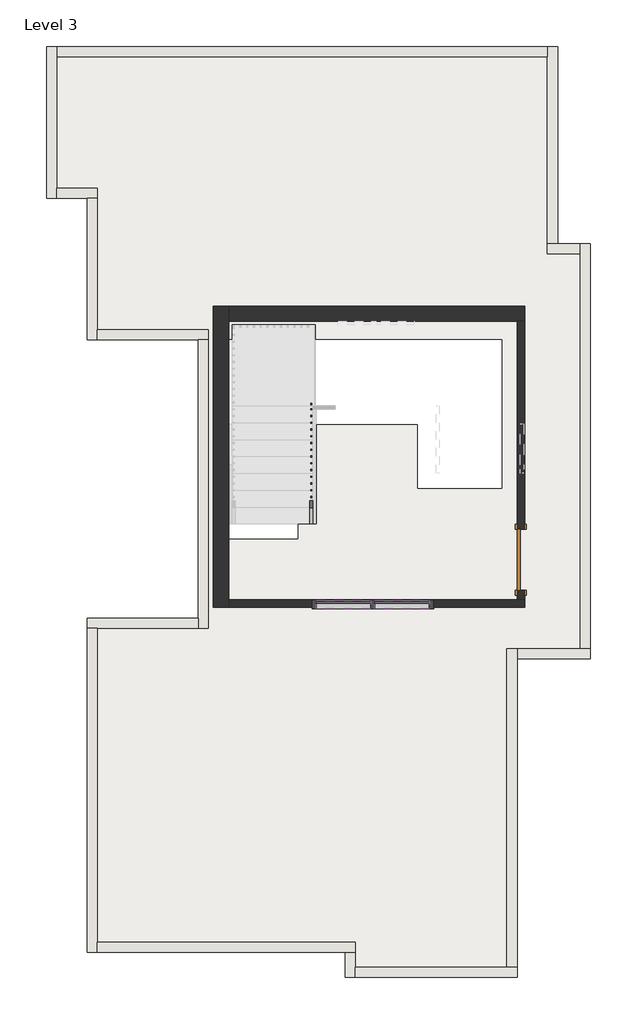
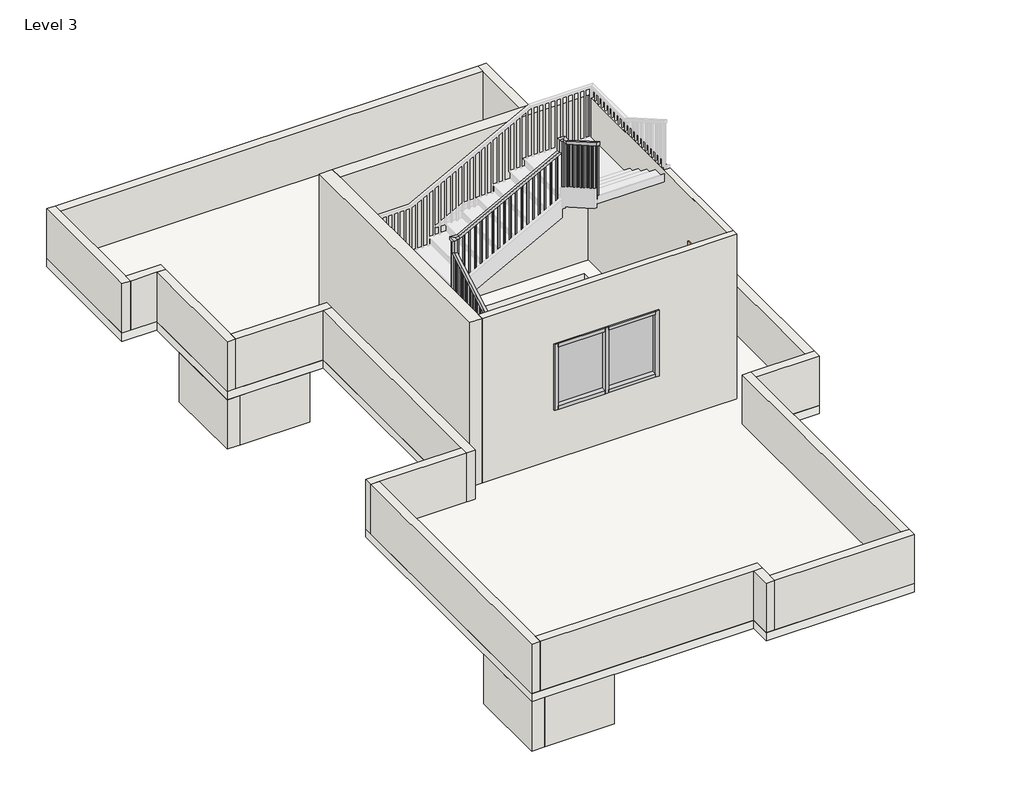
# One storey, part 1 of 2: 24 walls, 7 members, 2 plates, 1 door, 1 railing, 1 roof.
"""IFC4 building model written with IfcOpenShell, lengths in millimetres."""

from ifc_helpers import new_model, si_unit, frame, origin, place, context, project, spatial, polyline, outline, extrude, faceted_brep, transform, mapped, element, save
from components import single_flush_door_3_305aa2a5, member_75074519, member_2b49869a, member_c17f1be2, system_panel_glazed_d6173012

model = new_model("IFC4")

# Units and contexts
model_context = context("Model", 3, world=origin())
ifc_project = project(units=[si_unit("LENGTHUNIT", "METRE", prefix="MILLI")], contexts=[model_context])

# Site, building, storey
site = spatial("IfcSite", under=ifc_project)
building = spatial("IfcBuilding", under=site)
storey = spatial("IfcBuildingStorey", under=building, Name="Level 3", Elevation=6248.4)

# Door
placement = place(None, origin())
single_flush_door_3_shape = single_flush_door_3_305aa2a5(model_context)
element("IfcDoor", 1, ObjectType="Single-Flush : door 3'", at=placement, inside=storey, context=model_context, shape_type="MappedRepresentation", body=[
    mapped(single_flush_door_3_shape, transform((-36373.0566834, 12147.2118061, 6248.4), x_axis=(0.0, -1.0, 0.0), y_axis=(1.0, 0.0, 0.0), z_axis=(0.0, 0.0, 1.0))),
])

# Members
member_shape = member_75074519(model_context)
element("IfcMember", 2, ObjectType="Rectangular Mullion : 2.5\" x 5\" rectangular", at=placement, inside=storey, context=model_context, shape_type="MappedRepresentation", body=[
    mapped(member_shape, transform((-37687.5066834, 11472.9643297, 7162.8), x_axis=(1.0, 0.0, 0.0), y_axis=(0.0, -1.0, 0.0), z_axis=(0.0, 0.0, -1.0))),
])
element("IfcMember", 3, ObjectType="Rectangular Mullion : 2.5\" x 5\" rectangular", at=placement, inside=storey, context=model_context, shape_type="MappedRepresentation", body=[
    mapped(member_shape, transform((-39516.3066834, 11472.9643297, 8382.0), x_axis=(-1.0, 0.0, 0.0), y_axis=(0.0, -1.0, 0.0), z_axis=(0.0, 0.0, 1.0))),
])
member_2_shape = member_2b49869a(model_context)
element("IfcMember", 4, ObjectType="Rectangular Mullion : 2.5\" x 5\" rectangular", at=placement, inside=storey, context=model_context, shape_type="MappedRepresentation", body=[
    mapped(member_2_shape, transform((-38601.9066834, 11472.9643297, 7162.8), x_axis=(1.0, 0.0, 0.0), y_axis=(0.0, -1.0, 0.0), z_axis=(0.0, 0.0, -1.0))),
])
member_3_shape = member_c17f1be2(model_context)
element("IfcMember", 5, ObjectType="Rectangular Mullion : 2.5\" x 5\" rectangular", at=placement, inside=storey, context=model_context, shape_type="MappedRepresentation", body=[
    mapped(member_3_shape, transform((-37751.0066834, 11472.9643297, 8382.0), x_axis=(0.0, 0.0, 1.0), y_axis=(0.0, -1.0, 0.0), z_axis=(1.0, 0.0, 0.0))),
])
element("IfcMember", 6, ObjectType="Rectangular Mullion : 2.5\" x 5\" rectangular", at=placement, inside=storey, context=model_context, shape_type="MappedRepresentation", body=[
    mapped(member_3_shape, transform((-38633.6566834, 11472.9643297, 8382.0), x_axis=(0.0, 0.0, 1.0), y_axis=(0.0, -1.0, 0.0), z_axis=(1.0, 0.0, 0.0))),
])
element("IfcMember", 7, ObjectType="Rectangular Mullion : 2.5\" x 5\" rectangular", at=placement, inside=storey, context=model_context, shape_type="MappedRepresentation", body=[
    mapped(member_3_shape, transform((-39452.8066834, 11472.9643297, 7162.8), x_axis=(0.0, 0.0, -1.0), y_axis=(0.0, -1.0, 0.0), z_axis=(-1.0, 0.0, 0.0))),
])
element("IfcMember", 8, ObjectType="Rectangular Mullion : 2.5\" x 5\" rectangular", at=placement, inside=storey, context=model_context, shape_type="MappedRepresentation", body=[
    mapped(member_3_shape, transform((-38570.1566834, 11472.9643297, 7162.8), x_axis=(0.0, 0.0, -1.0), y_axis=(0.0, -1.0, 0.0), z_axis=(-1.0, 0.0, 0.0))),
])

# Plates
system_panel_glazed_shape = system_panel_glazed_d6173012(model_context)
element("IfcPlate", 9, ObjectType="System Panel : Glazed", at=placement, inside=storey, context=model_context, shape_type="MappedRepresentation", body=[
    mapped(system_panel_glazed_shape, transform((-39043.2316834, 11472.9643297, 7226.3), x_axis=(1.0, 0.0, 0.0), y_axis=(0.0, 1.0, 0.0), z_axis=(0.0, 0.0, 1.0))),
])
element("IfcPlate", 10, ObjectType="System Panel : Glazed", at=placement, inside=storey, context=model_context, shape_type="MappedRepresentation", body=[
    mapped(system_panel_glazed_shape, transform((-38160.5816834, 11472.9643297, 7226.3), x_axis=(1.0, 0.0, 0.0), y_axis=(0.0, 1.0, 0.0), z_axis=(0.0, 0.0, 1.0))),
])

# Railing
element("IfcRailing", 11, ObjectType="Handrail - Rectangular", at=placement, inside=storey, context=model_context, shape_type="SolidModel", body=[
    faceted_brep([(-39553.9146233, 12686.9618061, 7307.9428571), (-39553.9146233, 12686.9618061, 7249.4339009), (-39503.1146233, 12686.9618061, 7249.4339009), (-39503.1146233, 12686.9618061, 7307.9428571), (-39553.9146233, 14388.7618061, 8280.4), (-39553.9146233, 14439.5618061, 8250.9196152), (-39503.1146233, 14439.5618061, 8250.9196152), (-39503.1146233, 14388.7618061, 8280.4), (-39553.9146233, 14388.7618061, 8509.7257143), (-39553.9146233, 14439.5618061, 8458.9257143), (-39503.1146233, 14439.5618061, 8458.9257143), (-39503.1146233, 14388.7618061, 8509.7257143), (-39553.9146233, 14515.7618061, 8509.7257143), (-39553.9146233, 14515.7618061, 8458.9257143), (-39503.1146233, 14464.9618061, 8458.9257143), (-39503.1146233, 14464.9618061, 8509.7257143), (-39426.9146233, 14515.7618061, 8509.7257143), (-39414.2146233, 14515.7618061, 8458.9257143), (-39414.2146233, 14464.9618061, 8458.9257143), (-39426.9146233, 14464.9618061, 8509.7257143), (-37674.3146233, 14515.7618061, 9444.4457143), (-37623.5146233, 14515.7618061, 9413.9657143), (-37623.5146233, 14464.9618061, 9413.9657143), (-37674.3146233, 14464.9618061, 9444.4457143), (-37674.3146233, 14515.7618061, 9673.7714286), (-37623.5146233, 14515.7618061, 9622.9714286), (-37623.5146233, 14464.9618061, 9622.9714286), (-37674.3146233, 14464.9618061, 9673.7714286), (-37547.3146233, 14515.7618061, 9673.7714286), (-37547.3146233, 14515.7618061, 9622.9714286), (-37598.1146233, 14464.9618061, 9622.9714286), (-37598.1146233, 14464.9618061, 9673.7714286), (-37547.3146233, 14388.7618061, 9673.7714286), (-37547.3146233, 14375.2711327, 9622.9714286), (-37598.1146233, 14375.2711327, 9622.9714286), (-37598.1146233, 14388.7618061, 9673.7714286), (-37547.3146233, 13448.9618061, 10210.8), (-37598.1146233, 13448.9618061, 10210.8), (-37598.1146233, 13448.9618061, 10152.2910438), (-37547.3146233, 13448.9618061, 10152.2910438)], [[[0, 1, 2, 3]], [[1, 0, 4, 5]], [[2, 1, 5, 6]], [[3, 2, 6, 7]], [[0, 3, 7, 4]], [[5, 4, 8, 9]], [[6, 5, 9, 10]], [[7, 6, 10, 11]], [[4, 7, 11, 8]], [[9, 8, 12, 13]], [[10, 9, 13, 14]], [[11, 10, 14, 15]], [[8, 11, 15, 12]], [[13, 12, 16, 17]], [[14, 13, 17, 18]], [[15, 14, 18, 19]], [[12, 15, 19, 16]], [[17, 16, 20, 21]], [[18, 17, 21, 22]], [[19, 18, 22, 23]], [[16, 19, 23, 20]], [[21, 20, 24, 25]], [[22, 21, 25, 26]], [[23, 22, 26, 27]], [[20, 23, 27, 24]], [[25, 24, 28, 29]], [[26, 25, 29, 30]], [[27, 26, 30, 31]], [[24, 27, 31, 28]], [[29, 28, 32, 33]], [[30, 29, 33, 34]], [[31, 30, 34, 35]], [[28, 31, 35, 32]], [[36, 37, 38, 39]], [[33, 32, 36, 39]], [[34, 33, 39, 38]], [[35, 34, 38, 37]], [[32, 35, 37, 36]]]),
    extrude(outline(polyline([(13464.8368061, 10143.2196152), (13483.8868061, 10132.3339009), (13483.8868061, 9151.2571429), (13464.8368061, 9151.2571429), (13464.8368061, 10143.2196152)])), frame((-37582.2396233, 0.0, 0.0), z_axis=(1.0, 0.0, 0.0), x_axis=(0.0, 1.0, 0.0)), (0.0, 0.0, 1.0), 19.05),
    extrude(outline(polyline([(13566.4368061, 10085.1624723), (13585.4868061, 10074.2767581), (13585.4868061, 9151.2571429), (13566.4368061, 9151.2571429), (13566.4368061, 10085.1624723)])), frame((-37582.2396233, 0.0, 0.0), z_axis=(1.0, 0.0, 0.0), x_axis=(0.0, 1.0, 0.0)), (0.0, 0.0, 1.0), 19.05),
    extrude(outline(polyline([(13668.0368061, 10027.1053295), (13687.0868061, 10016.2196152), (13687.0868061, 9151.2571429), (13668.0368061, 9151.2571429), (13668.0368061, 10027.1053295)])), frame((-37582.2396233, 0.0, 0.0), z_axis=(1.0, 0.0, 0.0), x_axis=(0.0, 1.0, 0.0)), (0.0, 0.0, 1.0), 19.05),
    extrude(outline(polyline([(13769.6368061, 9969.0481866), (13788.6868061, 9958.1624723), (13788.6868061, 9006.1142857), (13769.6368061, 9006.1142857), (13769.6368061, 9969.0481866)])), frame((-37582.2396233, 0.0, 0.0), z_axis=(1.0, 0.0, 0.0), x_axis=(0.0, 1.0, 0.0)), (0.0, 0.0, 1.0), 19.05),
    extrude(outline(polyline([(13871.2368061, 9910.9910438), (13890.2868061, 9900.1053295), (13890.2868061, 9006.1142857), (13871.2368061, 9006.1142857), (13871.2368061, 9910.9910438)])), frame((-37582.2396233, 0.0, 0.0), z_axis=(1.0, 0.0, 0.0), x_axis=(0.0, 1.0, 0.0)), (0.0, 0.0, 1.0), 19.05),
    extrude(outline(polyline([(13972.8368061, 9852.9339009), (13991.8868061, 9842.0481866), (13991.8868061, 8860.9714286), (13972.8368061, 8860.9714286), (13972.8368061, 9852.9339009)])), frame((-37582.2396233, 0.0, 0.0), z_axis=(1.0, 0.0, 0.0), x_axis=(0.0, 1.0, 0.0)), (0.0, 0.0, 1.0), 19.05),
    extrude(outline(polyline([(14074.4368061, 9794.8767581), (14093.4868061, 9783.9910438), (14093.4868061, 8860.9714286), (14074.4368061, 8860.9714286), (14074.4368061, 9794.8767581)])), frame((-37582.2396233, 0.0, 0.0), z_axis=(1.0, 0.0, 0.0), x_axis=(0.0, 1.0, 0.0)), (0.0, 0.0, 1.0), 19.05),
    extrude(outline(polyline([(14176.0368061, 9736.8196152), (14195.0868061, 9725.9339009), (14195.0868061, 8860.9714286), (14176.0368061, 8860.9714286), (14176.0368061, 9736.8196152)])), frame((-37582.2396233, 0.0, 0.0), z_axis=(1.0, 0.0, 0.0), x_axis=(0.0, 1.0, 0.0)), (0.0, 0.0, 1.0), 19.05),
    extrude(outline(polyline([(14277.6368061, 9678.7624723), (14296.6868061, 9667.8767581), (14296.6868061, 8715.8285714), (14277.6368061, 8715.8285714), (14277.6368061, 9678.7624723)])), frame((-37582.2396233, 0.0, 0.0), z_axis=(1.0, 0.0, 0.0), x_axis=(0.0, 1.0, 0.0)), (0.0, 0.0, 1.0), 19.05),
    extrude(outline(polyline([(14379.2368061, 9620.7053295), (14398.2868061, 9609.8196152), (14398.2868061, 8715.8285714), (14379.2368061, 8715.8285714), (14379.2368061, 9620.7053295)])), frame((-37582.2396233, 0.0, 0.0), z_axis=(1.0, 0.0, 0.0), x_axis=(0.0, 1.0, 0.0)), (0.0, 0.0, 1.0), 19.05),
    extrude(outline(polyline([(-37607.6396233, 14480.8368061), (-37607.6396233, 14499.8868061), (-37588.5896233, 14499.8868061), (-37588.5896233, 14480.8368061), (-37607.6396233, 14480.8368061)])), frame((0.0, 0.0, 8570.6857143), z_axis=(0.0, 0.0, 1.0), x_axis=(1.0, 0.0, 0.0)), (0.0, 0.0, 1.0), 1052.2857143),
    extrude(outline(polyline([(9378.4057143, -37690.1896233), (9368.2457143, -37709.2396233), (8425.5428571, -37709.2396233), (8425.5428571, -37690.1896233), (9378.4057143, -37690.1896233)])), frame((0.0, 14480.8368061, 0.0), z_axis=(0.0, 1.0, 0.0), x_axis=(0.0, 0.0, 1.0)), (0.0, 0.0, 1.0), 19.05),
    extrude(outline(polyline([(9324.2190476, -37791.7896233), (9314.0590476, -37810.8396233), (8425.5428571, -37810.8396233), (8425.5428571, -37791.7896233), (9324.2190476, -37791.7896233)])), frame((0.0, 14480.8368061, 0.0), z_axis=(0.0, 1.0, 0.0), x_axis=(0.0, 0.0, 1.0)), (0.0, 0.0, 1.0), 19.05),
    extrude(outline(polyline([(9270.032381, -37893.3896233), (9259.872381, -37912.4396233), (8280.4, -37912.4396233), (8280.4, -37893.3896233), (9270.032381, -37893.3896233)])), frame((0.0, 14480.8368061, 0.0), z_axis=(0.0, 1.0, 0.0), x_axis=(0.0, 0.0, 1.0)), (0.0, 0.0, 1.0), 19.05),
    extrude(outline(polyline([(9215.8457143, -37994.9896233), (9205.6857143, -38014.0396233), (8280.4, -38014.0396233), (8280.4, -37994.9896233), (9215.8457143, -37994.9896233)])), frame((0.0, 14480.8368061, 0.0), z_axis=(0.0, 1.0, 0.0), x_axis=(0.0, 0.0, 1.0)), (0.0, 0.0, 1.0), 19.05),
    extrude(outline(polyline([(9161.6590476, -38096.5896233), (9151.4990476, -38115.6396233), (8280.4, -38115.6396233), (8280.4, -38096.5896233), (9161.6590476, -38096.5896233)])), frame((0.0, 14480.8368061, 0.0), z_axis=(0.0, 1.0, 0.0), x_axis=(0.0, 0.0, 1.0)), (0.0, 0.0, 1.0), 19.05),
    extrude(outline(polyline([(9107.472381, -38198.1896233), (9097.312381, -38217.2396233), (8135.2571429, -38217.2396233), (8135.2571429, -38198.1896233), (9107.472381, -38198.1896233)])), frame((0.0, 14480.8368061, 0.0), z_axis=(0.0, 1.0, 0.0), x_axis=(0.0, 0.0, 1.0)), (0.0, 0.0, 1.0), 19.05),
    extrude(outline(polyline([(9053.2857143, -38299.7896233), (9043.1257143, -38318.8396233), (8135.2571429, -38318.8396233), (8135.2571429, -38299.7896233), (9053.2857143, -38299.7896233)])), frame((0.0, 14480.8368061, 0.0), z_axis=(0.0, 1.0, 0.0), x_axis=(0.0, 0.0, 1.0)), (0.0, 0.0, 1.0), 19.05),
    extrude(outline(polyline([(8999.0990476, -38401.3896233), (8988.9390476, -38420.4396233), (8135.2571429, -38420.4396233), (8135.2571429, -38401.3896233), (8999.0990476, -38401.3896233)])), frame((0.0, 14480.8368061, 0.0), z_axis=(0.0, 1.0, 0.0), x_axis=(0.0, 0.0, 1.0)), (0.0, 0.0, 1.0), 19.05),
    extrude(outline(polyline([(8944.912381, -38502.9896233), (8934.752381, -38522.0396233), (7990.1142857, -38522.0396233), (7990.1142857, -38502.9896233), (8944.912381, -38502.9896233)])), frame((0.0, 14480.8368061, 0.0), z_axis=(0.0, 1.0, 0.0), x_axis=(0.0, 0.0, 1.0)), (0.0, 0.0, 1.0), 19.05),
    extrude(outline(polyline([(8890.7257143, -38604.5896233), (8880.5657143, -38623.6396233), (7990.1142857, -38623.6396233), (7990.1142857, -38604.5896233), (8890.7257143, -38604.5896233)])), frame((0.0, 14480.8368061, 0.0), z_axis=(0.0, 1.0, 0.0), x_axis=(0.0, 0.0, 1.0)), (0.0, 0.0, 1.0), 19.05),
    extrude(outline(polyline([(8836.5390476, -38706.1896233), (8826.3790476, -38725.2396233), (7844.9714286, -38725.2396233), (7844.9714286, -38706.1896233), (8836.5390476, -38706.1896233)])), frame((0.0, 14480.8368061, 0.0), z_axis=(0.0, 1.0, 0.0), x_axis=(0.0, 0.0, 1.0)), (0.0, 0.0, 1.0), 19.05),
    extrude(outline(polyline([(8782.352381, -38807.7896233), (8772.192381, -38826.8396233), (7844.9714286, -38826.8396233), (7844.9714286, -38807.7896233), (8782.352381, -38807.7896233)])), frame((0.0, 14480.8368061, 0.0), z_axis=(0.0, 1.0, 0.0), x_axis=(0.0, 0.0, 1.0)), (0.0, 0.0, 1.0), 19.05),
    extrude(outline(polyline([(8728.1657143, -38909.3896233), (8718.0057143, -38928.4396233), (7844.9714286, -38928.4396233), (7844.9714286, -38909.3896233), (8728.1657143, -38909.3896233)])), frame((0.0, 14480.8368061, 0.0), z_axis=(0.0, 1.0, 0.0), x_axis=(0.0, 0.0, 1.0)), (0.0, 0.0, 1.0), 19.05),
    extrude(outline(polyline([(8673.9790476, -39010.9896233), (8663.8190476, -39030.0396233), (7699.8285714, -39030.0396233), (7699.8285714, -39010.9896233), (8673.9790476, -39010.9896233)])), frame((0.0, 14480.8368061, 0.0), z_axis=(0.0, 1.0, 0.0), x_axis=(0.0, 0.0, 1.0)), (0.0, 0.0, 1.0), 19.05),
    extrude(outline(polyline([(8619.792381, -39112.5896233), (8609.632381, -39131.6396233), (7699.8285714, -39131.6396233), (7699.8285714, -39112.5896233), (8619.792381, -39112.5896233)])), frame((0.0, 14480.8368061, 0.0), z_axis=(0.0, 1.0, 0.0), x_axis=(0.0, 0.0, 1.0)), (0.0, 0.0, 1.0), 19.05),
    extrude(outline(polyline([(8565.6057143, -39214.1896233), (8555.4457143, -39233.2396233), (7699.8285714, -39233.2396233), (7699.8285714, -39214.1896233), (8565.6057143, -39214.1896233)])), frame((0.0, 14480.8368061, 0.0), z_axis=(0.0, 1.0, 0.0), x_axis=(0.0, 0.0, 1.0)), (0.0, 0.0, 1.0), 19.05),
    extrude(outline(polyline([(8511.4190476, -39315.7896233), (8501.2590476, -39334.8396233), (7554.6857143, -39334.8396233), (7554.6857143, -39315.7896233), (8511.4190476, -39315.7896233)])), frame((0.0, 14480.8368061, 0.0), z_axis=(0.0, 1.0, 0.0), x_axis=(0.0, 0.0, 1.0)), (0.0, 0.0, 1.0), 19.05),
    extrude(outline(polyline([(8457.232381, -39417.3896233), (8447.072381, -39436.4396233), (7554.6857143, -39436.4396233), (7554.6857143, -39417.3896233), (8457.232381, -39417.3896233)])), frame((0.0, 14480.8368061, 0.0), z_axis=(0.0, 1.0, 0.0), x_axis=(0.0, 0.0, 1.0)), (0.0, 0.0, 1.0), 19.05),
    extrude(outline(polyline([(-39518.9896233, 14404.6368061), (-39538.0396233, 14404.6368061), (-39538.0396233, 14423.6868061), (-39518.9896233, 14423.6868061), (-39518.9896233, 14404.6368061)])), frame((0.0, 0.0, 7264.4), z_axis=(0.0, 0.0, 1.0), x_axis=(1.0, 0.0, 0.0)), (0.0, 0.0, 1.0), 1194.5257143),
    extrude(outline(polyline([(14303.0368061, 8172.9053295), (14322.0868061, 8183.7910438), (14322.0868061, 7264.4), (14303.0368061, 7264.4), (14303.0368061, 8172.9053295)])), frame((-39538.0396233, 0.0, 0.0), z_axis=(1.0, 0.0, 0.0), x_axis=(0.0, 1.0, 0.0)), (0.0, 0.0, 1.0), 19.05),
    extrude(outline(polyline([(14201.4368061, 8114.8481866), (14220.4868061, 8125.7339009), (14220.4868061, 7264.4), (14201.4368061, 7264.4), (14201.4368061, 8114.8481866)])), frame((-39538.0396233, 0.0, 0.0), z_axis=(1.0, 0.0, 0.0), x_axis=(0.0, 1.0, 0.0)), (0.0, 0.0, 1.0), 19.05),
    extrude(outline(polyline([(14099.8368061, 8056.7910438), (14118.8868061, 8067.6767581), (14118.8868061, 7119.2571429), (14099.8368061, 7119.2571429), (14099.8368061, 8056.7910438)])), frame((-39538.0396233, 0.0, 0.0), z_axis=(1.0, 0.0, 0.0), x_axis=(0.0, 1.0, 0.0)), (0.0, 0.0, 1.0), 19.05),
    extrude(outline(polyline([(13998.2368061, 7998.7339009), (14017.2868061, 8009.6196152), (14017.2868061, 7119.2571429), (13998.2368061, 7119.2571429), (13998.2368061, 7998.7339009)])), frame((-39538.0396233, 0.0, 0.0), z_axis=(1.0, 0.0, 0.0), x_axis=(0.0, 1.0, 0.0)), (0.0, 0.0, 1.0), 19.05),
    extrude(outline(polyline([(13896.6368061, 7940.6767581), (13915.6868061, 7951.5624723), (13915.6868061, 6974.1142857), (13896.6368061, 6974.1142857), (13896.6368061, 7940.6767581)])), frame((-39538.0396233, 0.0, 0.0), z_axis=(1.0, 0.0, 0.0), x_axis=(0.0, 1.0, 0.0)), (0.0, 0.0, 1.0), 19.05),
    extrude(outline(polyline([(13795.0368061, 7882.6196152), (13814.0868061, 7893.5053295), (13814.0868061, 6974.1142857), (13795.0368061, 6974.1142857), (13795.0368061, 7882.6196152)])), frame((-39538.0396233, 0.0, 0.0), z_axis=(1.0, 0.0, 0.0), x_axis=(0.0, 1.0, 0.0)), (0.0, 0.0, 1.0), 19.05),
    extrude(outline(polyline([(13693.4368061, 7824.5624723), (13712.4868061, 7835.4481866), (13712.4868061, 6974.1142857), (13693.4368061, 6974.1142857), (13693.4368061, 7824.5624723)])), frame((-39538.0396233, 0.0, 0.0), z_axis=(1.0, 0.0, 0.0), x_axis=(0.0, 1.0, 0.0)), (0.0, 0.0, 1.0), 19.05),
    extrude(outline(polyline([(13591.8368061, 7766.5053295), (13610.8868061, 7777.3910438), (13610.8868061, 6828.9714286), (13591.8368061, 6828.9714286), (13591.8368061, 7766.5053295)])), frame((-39538.0396233, 0.0, 0.0), z_axis=(1.0, 0.0, 0.0), x_axis=(0.0, 1.0, 0.0)), (0.0, 0.0, 1.0), 19.05),
    extrude(outline(polyline([(13490.2368061, 7708.4481866), (13509.2868061, 7719.3339009), (13509.2868061, 6828.9714286), (13490.2368061, 6828.9714286), (13490.2368061, 7708.4481866)])), frame((-39538.0396233, 0.0, 0.0), z_axis=(1.0, 0.0, 0.0), x_axis=(0.0, 1.0, 0.0)), (0.0, 0.0, 1.0), 19.05),
    extrude(outline(polyline([(13388.6368061, 7650.3910438), (13407.6868061, 7661.2767581), (13407.6868061, 6683.8285714), (13388.6368061, 6683.8285714), (13388.6368061, 7650.3910438)])), frame((-39538.0396233, 0.0, 0.0), z_axis=(1.0, 0.0, 0.0), x_axis=(0.0, 1.0, 0.0)), (0.0, 0.0, 1.0), 19.05),
    extrude(outline(polyline([(13287.0368061, 7592.3339009), (13306.0868061, 7603.2196152), (13306.0868061, 6683.8285714), (13287.0368061, 6683.8285714), (13287.0368061, 7592.3339009)])), frame((-39538.0396233, 0.0, 0.0), z_axis=(1.0, 0.0, 0.0), x_axis=(0.0, 1.0, 0.0)), (0.0, 0.0, 1.0), 19.05),
    extrude(outline(polyline([(13185.4368061, 7534.2767581), (13204.4868061, 7545.1624723), (13204.4868061, 6683.8285714), (13185.4368061, 6683.8285714), (13185.4368061, 7534.2767581)])), frame((-39538.0396233, 0.0, 0.0), z_axis=(1.0, 0.0, 0.0), x_axis=(0.0, 1.0, 0.0)), (0.0, 0.0, 1.0), 19.05),
    extrude(outline(polyline([(13083.8368061, 7476.2196152), (13102.8868061, 7487.1053295), (13102.8868061, 6538.6857143), (13083.8368061, 6538.6857143), (13083.8368061, 7476.2196152)])), frame((-39538.0396233, 0.0, 0.0), z_axis=(1.0, 0.0, 0.0), x_axis=(0.0, 1.0, 0.0)), (0.0, 0.0, 1.0), 19.05),
    extrude(outline(polyline([(12982.2368061, 7418.1624723), (13001.2868061, 7429.0481866), (13001.2868061, 6538.6857143), (12982.2368061, 6538.6857143), (12982.2368061, 7418.1624723)])), frame((-39538.0396233, 0.0, 0.0), z_axis=(1.0, 0.0, 0.0), x_axis=(0.0, 1.0, 0.0)), (0.0, 0.0, 1.0), 19.05),
    extrude(outline(polyline([(12880.6368061, 7360.1053295), (12899.6868061, 7370.9910438), (12899.6868061, 6393.5428571), (12880.6368061, 6393.5428571), (12880.6368061, 7360.1053295)])), frame((-39538.0396233, 0.0, 0.0), z_axis=(1.0, 0.0, 0.0), x_axis=(0.0, 1.0, 0.0)), (0.0, 0.0, 1.0), 19.05),
    extrude(outline(polyline([(12779.0368061, 7302.0481866), (12798.0868061, 7312.9339009), (12798.0868061, 6393.5428571), (12779.0368061, 6393.5428571), (12779.0368061, 7302.0481866)])), frame((-39538.0396233, 0.0, 0.0), z_axis=(1.0, 0.0, 0.0), x_axis=(0.0, 1.0, 0.0)), (0.0, 0.0, 1.0), 19.05),
    extrude(outline(polyline([(-37582.2396233, 14480.8368061), (-37582.2396233, 14499.8868061), (-37563.1896233, 14499.8868061), (-37563.1896233, 14480.8368061), (-37582.2396233, 14480.8368061)])), frame((0.0, 0.0, 8570.6857143), z_axis=(0.0, 0.0, 1.0), x_axis=(1.0, 0.0, 0.0)), (0.0, 0.0, 1.0), 1052.2857143),
    extrude(outline(polyline([(-39518.9896233, 14480.8368061), (-39538.0396233, 14480.8368061), (-39538.0396233, 14499.8868061), (-39518.9896233, 14499.8868061), (-39518.9896233, 14480.8368061)])), frame((0.0, 0.0, 7409.5428571), z_axis=(0.0, 0.0, 1.0), x_axis=(1.0, 0.0, 0.0)), (0.0, 0.0, 1.0), 1049.3828571),
    extrude(outline(polyline([(13448.9618061, 10152.2910438), (13468.0118061, 10141.4053295), (13468.0118061, 9151.2571429), (13448.9618061, 9151.2571429), (13448.9618061, 10152.2910438)])), frame((-37582.2396233, 0.0, 0.0), z_axis=(1.0, 0.0, 0.0), x_axis=(0.0, 1.0, 0.0)), (0.0, 0.0, 1.0), 19.05),
    extrude(outline(polyline([(12686.9618061, 7249.4339009), (12706.0118061, 7260.3196152), (12706.0118061, 6393.5428571), (12686.9618061, 6393.5428571), (12686.9618061, 7249.4339009)])), frame((-39538.0396233, 0.0, 0.0), z_axis=(1.0, 0.0, 0.0), x_axis=(0.0, 1.0, 0.0)), (0.0, 0.0, 1.0), 19.05),
])

# Roof
element("IfcRoof", 12, ObjectType="ROOF 6\"", at=placement, inside=storey, context=model_context, shape_type="SweptSolid", body=[
    extrude(outline(polyline([(-42906.7146233, 15456.5864709), (-42906.7146233, 17590.1864709), (-43516.3146233, 17590.1864709), (-43516.3146233, 19876.1864709), (-35820.1146233, 19876.1864709), (-35820.1146233, 16904.3864709), (-35324.8146233, 16904.3864709), (-35324.8146233, 10655.9864709), (-36429.7146233, 10655.9864709), (-36429.7146233, 5855.3080647), (-39020.5146233, 5855.3080647), (-39020.5146233, 6236.3864709), (-42906.7146233, 6236.3864709), (-42906.7146233, 11265.5864709), (-41230.3146233, 11265.5864709), (-41230.3146233, 15456.5864709), (-42906.7146233, 15456.5864709)]), holes=[polyline([(-36658.3146233, 15456.5864709), (-41001.7146233, 15456.5864709), (-41001.7146233, 12459.3864709), (-39731.7146233, 12459.3864709), (-39731.7146233, 14186.5864709), (-37928.3146233, 14186.5864709), (-37928.3146233, 13221.3864709), (-36658.3146233, 13221.3864709), (-36658.3146233, 15456.5864709)])]), frame((0.0, 0.0, 6096.0), z_axis=(0.0, 0.0, 1.0), x_axis=(1.0, 0.0, 0.0)), (0.0, 0.0, 1.0), 152.4),
])

# Walls
element("IfcWall", 13, ObjectType="Generic - 5\"", at=placement, inside=storey, context=model_context, shape_type="Brep", body=[
    faceted_brep([(-40773.1146233, 11429.6618061, 6248.4), (-36315.9066834, 11429.6618061, 6248.4), (-36315.9066834, 11429.6618061, 9296.4), (-40773.1146233, 11429.6618061, 9296.4), (-39516.3066834, 11429.6618061, 7162.8), (-39516.3066834, 11429.6618061, 8382.0), (-37687.5066834, 11429.6618061, 8382.0), (-37687.5066834, 11429.6618061, 7162.8), (-36315.9066834, 11543.9618061, 6248.4), (-36430.2066834, 11543.9618061, 6248.4), (-40773.1146233, 11543.9618061, 6248.4), (-40773.1146233, 11543.9618061, 9296.4), (-36430.2066834, 11543.9618061, 9296.4), (-36315.9066834, 11543.9618061, 9296.4), (-39516.3066834, 11543.9618061, 8382.0), (-39516.3066834, 11543.9618061, 7162.8), (-37687.5066834, 11543.9618061, 7162.8), (-37687.5066834, 11543.9618061, 8382.0)], [[[0, 1, 2, 3], [4, 5, 6, 7]], [[8, 9, 10, 11, 12, 13], [14, 15, 16, 17]], [[1, 0, 10, 9, 8]], [[2, 1, 8, 13]], [[0, 3, 11, 10]], [[4, 15, 14, 5]], [[5, 14, 17, 6]], [[6, 17, 16, 7]], [[15, 4, 7, 16]], [[3, 2, 13, 12, 11]]]),
])
element("IfcWall", 14, ObjectType="Generic - 5\"", at=placement, inside=storey, context=model_context, shape_type="Brep", body=[
    faceted_brep([(-36315.9066834, 11543.9618061, 6248.4), (-36315.9066834, 11690.0118061, 6248.4), (-36315.9066834, 11690.0118061, 8382.0), (-36315.9066834, 12604.4118061, 8382.0), (-36315.9066834, 12604.4118061, 6248.4), (-36315.9066834, 15734.9618061, 6248.4), (-36315.9066834, 15734.9618061, 9296.4), (-36315.9066834, 11543.9618061, 9296.4), (-36430.2066834, 11690.0118061, 8382.0), (-36430.2066834, 11690.0118061, 6248.4), (-36430.2066834, 11543.9618061, 6248.4), (-36430.2066834, 11543.9618061, 9296.4), (-36430.2066834, 15734.9618061, 9296.4), (-36430.2066834, 15734.9618061, 6248.4), (-36430.2066834, 12604.4118061, 6248.4), (-36430.2066834, 12604.4118061, 8382.0), (-36429.7146233, 11543.9618061, 9296.4), (-36429.7146233, 15734.9618061, 9296.4), (-36429.7146233, 13448.9618061, 9296.4)], [[[0, 1, 2, 3, 4, 5, 6, 7]], [[8, 9, 10, 11, 12, 13, 14, 15]], [[14, 13, 5, 4]], [[10, 9, 1, 0]], [[0, 7, 16, 11, 10]], [[6, 5, 13, 12, 17]], [[2, 1, 9, 8]], [[3, 2, 8, 15]], [[4, 3, 15, 14]], [[7, 6, 17, 18, 16]], [[17, 12, 11, 16, 18]]]),
])
element("IfcWall", 15, ObjectType="PARAPET WALL", at=placement, inside=storey, context=model_context, shape_type="Brep", body=[
    faceted_brep([(-43516.3146233, 19876.1864709, 6248.4), (-43516.3146233, 17590.1864709, 6248.4), (-43516.3146233, 17590.1864709, 7162.8), (-43516.3146233, 19876.1864709, 7162.8), (-43363.9146233, 19876.1864709, 6248.4), (-43363.9146233, 19876.1864709, 7162.8), (-43363.9146233, 19723.7864709, 7162.8), (-43363.9146233, 17742.5864709, 7162.8), (-43363.9146233, 17590.1864709, 7162.8), (-43363.9146233, 17590.1864709, 6248.4), (-43363.9146233, 17742.5864709, 6248.4), (-43363.9146233, 19723.7864709, 6248.4)], [[[0, 1, 2, 3]], [[4, 5, 6, 7, 8, 9, 10, 11]], [[1, 0, 4, 11, 10, 9]], [[3, 2, 8, 7, 6, 5]], [[2, 1, 9, 8]], [[0, 3, 5, 4]]]),
])
element("IfcWall", 16, ObjectType="PARAPET WALL", at=placement, inside=storey, context=model_context, shape_type="Brep", body=[
    faceted_brep([(-43363.9146233, 17590.1864709, 6248.4), (-42906.7146233, 17590.1864709, 6248.4), (-42754.3146233, 17590.1864709, 6248.4), (-42754.3146233, 17590.1864709, 7162.8), (-42906.7146233, 17590.1864709, 7162.8), (-43363.9146233, 17590.1864709, 7162.8), (-43363.9146233, 17742.5864709, 6248.4), (-43363.9146233, 17742.5864709, 7162.8), (-42754.3146233, 17742.5864709, 7162.8), (-42754.3146233, 17742.5864709, 6248.4)], [[[0, 1, 2, 3, 4, 5]], [[6, 7, 8, 9]], [[2, 1, 0, 6, 9]], [[5, 4, 3, 8, 7]], [[0, 5, 7, 6]], [[3, 2, 9, 8]]]),
])
element("IfcWall", 17, ObjectType="PARAPET WALL", at=placement, inside=storey, context=model_context, shape_type="Brep", body=[
    faceted_brep([(-42906.7146233, 17590.1864709, 6248.4), (-42906.7146233, 15456.5864709, 6248.4), (-42906.7146233, 15456.5864709, 7162.8), (-42906.7146233, 17590.1864709, 7162.8), (-42754.3146233, 17590.1864709, 6248.4), (-42754.3146233, 17590.1864709, 7162.8), (-42754.3146233, 15608.9864709, 7162.8), (-42754.3146233, 15456.5864709, 7162.8), (-42754.3146233, 15456.5864709, 6248.4), (-42754.3146233, 15608.9864709, 6248.4)], [[[0, 1, 2, 3]], [[4, 5, 6, 7, 8, 9]], [[1, 0, 4, 9, 8]], [[3, 2, 7, 6, 5]], [[0, 3, 5, 4]], [[2, 1, 8, 7]]]),
])
element("IfcWall", 18, ObjectType="PARAPET WALL", at=placement, inside=storey, context=model_context, shape_type="Brep", body=[
    faceted_brep([(-42754.3146233, 15456.5864709, 6248.4), (-41230.3146233, 15456.5864709, 6248.4), (-41077.9146233, 15456.5864709, 6248.4), (-41077.9146233, 15456.5864709, 7162.8), (-41230.3146233, 15456.5864709, 7162.8), (-42754.3146233, 15456.5864709, 7162.8), (-42754.3146233, 15608.9864709, 6248.4), (-42754.3146233, 15608.9864709, 7162.8), (-41077.9146233, 15608.9864709, 7162.8), (-41077.9146233, 15608.9864709, 6248.4)], [[[0, 1, 2, 3, 4, 5]], [[6, 7, 8, 9]], [[2, 1, 0, 6, 9]], [[5, 4, 3, 8, 7]], [[0, 5, 7, 6]], [[3, 2, 9, 8]]]),
])
element("IfcWall", 19, ObjectType="PARAPET WALL", at=placement, inside=storey, context=model_context, shape_type="Brep", body=[
    faceted_brep([(-41230.3146233, 15456.5864709, 6248.4), (-41230.3146233, 11265.5864709, 6248.4), (-41230.3146233, 11113.1864709, 6248.4), (-41230.3146233, 11113.1864709, 7162.8), (-41230.3146233, 11265.5864709, 7162.8), (-41230.3146233, 15456.5864709, 7162.8), (-41077.9146233, 15456.5864709, 6248.4), (-41077.9146233, 15456.5864709, 7162.8), (-41077.9146233, 11113.1864709, 7162.8), (-41077.9146233, 11113.1864709, 6248.4)], [[[0, 1, 2, 3, 4, 5]], [[6, 7, 8, 9]], [[2, 1, 0, 6, 9]], [[5, 4, 3, 8, 7]], [[0, 5, 7, 6]], [[3, 2, 9, 8]]]),
])
element("IfcWall", 20, ObjectType="PARAPET WALL", at=placement, inside=storey, context=model_context, shape_type="Brep", body=[
    faceted_brep([(-41230.3146233, 11265.5864709, 6248.4), (-42906.7146233, 11265.5864709, 6248.4), (-42906.7146233, 11265.5864709, 7162.8), (-41230.3146233, 11265.5864709, 7162.8), (-41230.3146233, 11113.1864709, 6248.4), (-41230.3146233, 11113.1864709, 7162.8), (-42754.3146233, 11113.1864709, 7162.8), (-42906.7146233, 11113.1864709, 7162.8), (-42906.7146233, 11113.1864709, 6248.4), (-42754.3146233, 11113.1864709, 6248.4)], [[[0, 1, 2, 3]], [[4, 5, 6, 7, 8, 9]], [[1, 0, 4, 9, 8]], [[3, 2, 7, 6, 5]], [[0, 3, 5, 4]], [[2, 1, 8, 7]]]),
])
element("IfcWall", 21, ObjectType="PARAPET WALL", at=placement, inside=storey, context=model_context, shape_type="Brep", body=[
    faceted_brep([(-42906.7146233, 11113.1864709, 6248.4), (-42906.7146233, 6236.3864709, 6248.4), (-42906.7146233, 6236.3864709, 7162.8), (-42906.7146233, 11113.1864709, 7162.8), (-42754.3146233, 11113.1864709, 6248.4), (-42754.3146233, 11113.1864709, 7162.8), (-42754.3146233, 6388.7864709, 7162.8), (-42754.3146233, 6236.3864709, 7162.8), (-42754.3146233, 6236.3864709, 6248.4), (-42754.3146233, 6388.7864709, 6248.4)], [[[0, 1, 2, 3]], [[4, 5, 6, 7, 8, 9]], [[1, 0, 4, 9, 8]], [[3, 2, 7, 6, 5]], [[0, 3, 5, 4]], [[2, 1, 8, 7]]]),
])
element("IfcWall", 22, ObjectType="PARAPET WALL", at=placement, inside=storey, context=model_context, shape_type="Brep", body=[
    faceted_brep([(-42754.3146233, 6236.3864709, 6248.4), (-39020.5146233, 6236.3864709, 6248.4), (-38868.1146233, 6236.3864709, 6248.4), (-38868.1146233, 6236.3864709, 7162.8), (-39020.5146233, 6236.3864709, 7162.8), (-42754.3146233, 6236.3864709, 7162.8), (-42754.3146233, 6388.7864709, 6248.4), (-42754.3146233, 6388.7864709, 7162.8), (-38868.1146233, 6388.7864709, 7162.8), (-38868.1146233, 6388.7864709, 6248.4)], [[[0, 1, 2, 3, 4, 5]], [[6, 7, 8, 9]], [[2, 1, 0, 6, 9]], [[5, 4, 3, 8, 7]], [[0, 5, 7, 6]], [[3, 2, 9, 8]]]),
])
element("IfcWall", 23, ObjectType="PARAPET WALL", at=placement, inside=storey, context=model_context, shape_type="Brep", body=[
    faceted_brep([(-39020.5146233, 6236.3864709, 6248.4), (-39020.5146233, 5855.3080647, 6248.4), (-39020.5146233, 5855.3080647, 7162.8), (-39020.5146233, 6236.3864709, 7162.8), (-38868.1146233, 6236.3864709, 6248.4), (-38868.1146233, 6236.3864709, 7162.8), (-38868.1146233, 6007.7080647, 7162.8), (-38868.1146233, 5855.3080647, 7162.8), (-38868.1146233, 5855.3080647, 6248.4), (-38868.1146233, 6007.7080647, 6248.4)], [[[0, 1, 2, 3]], [[4, 5, 6, 7, 8, 9]], [[1, 0, 4, 9, 8]], [[3, 2, 7, 6, 5]], [[0, 3, 5, 4]], [[2, 1, 8, 7]]]),
])
element("IfcWall", 24, ObjectType="PARAPET WALL", at=placement, inside=storey, context=model_context, shape_type="Brep", body=[
    faceted_brep([(-38868.1146233, 5855.3080647, 6248.4), (-36429.7146233, 5855.3080647, 6248.4), (-36429.7146233, 5855.3080647, 7162.8), (-38868.1146233, 5855.3080647, 7162.8), (-38868.1146233, 6007.7080647, 6248.4), (-38868.1146233, 6007.7080647, 7162.8), (-36582.1146233, 6007.7080647, 7162.8), (-36429.7146233, 6007.7080647, 7162.8), (-36429.7146233, 6007.7080647, 6248.4), (-36582.1146233, 6007.7080647, 6248.4)], [[[0, 1, 2, 3]], [[4, 5, 6, 7, 8, 9]], [[1, 0, 4, 9, 8]], [[3, 2, 7, 6, 5]], [[0, 3, 5, 4]], [[2, 1, 8, 7]]]),
])
element("IfcWall", 25, ObjectType="PARAPET WALL", at=placement, inside=storey, context=model_context, shape_type="Brep", body=[
    faceted_brep([(-36429.7146233, 6007.7080647, 6248.4), (-36429.7146233, 10655.9864709, 6248.4), (-36429.7146233, 10808.3864709, 6248.4), (-36429.7146233, 10808.3864709, 7162.8), (-36429.7146233, 10655.9864709, 7162.8), (-36429.7146233, 6007.7080647, 7162.8), (-36582.1146233, 6007.7080647, 6248.4), (-36582.1146233, 6007.7080647, 7162.8), (-36582.1146233, 10808.3864709, 7162.8), (-36582.1146233, 10808.3864709, 6248.4)], [[[0, 1, 2, 3, 4, 5]], [[6, 7, 8, 9]], [[2, 1, 0, 6, 9]], [[5, 4, 3, 8, 7]], [[0, 5, 7, 6]], [[3, 2, 9, 8]]]),
])
element("IfcWall", 26, ObjectType="PARAPET WALL", at=placement, inside=storey, context=model_context, shape_type="Brep", body=[
    faceted_brep([(-36429.7146233, 10655.9864709, 6248.4), (-35324.8146233, 10655.9864709, 6248.4), (-35324.8146233, 10655.9864709, 7162.8), (-36429.7146233, 10655.9864709, 7162.8), (-36429.7146233, 10808.3864709, 6248.4), (-36429.7146233, 10808.3864709, 7162.8), (-35477.2146233, 10808.3864709, 7162.8), (-35324.8146233, 10808.3864709, 7162.8), (-35324.8146233, 10808.3864709, 6248.4), (-35477.2146233, 10808.3864709, 6248.4)], [[[0, 1, 2, 3]], [[4, 5, 6, 7, 8, 9]], [[1, 0, 4, 9, 8]], [[3, 2, 7, 6, 5]], [[0, 3, 5, 4]], [[2, 1, 8, 7]]]),
])
element("IfcWall", 27, ObjectType="PARAPET WALL", at=placement, inside=storey, context=model_context, shape_type="Brep", body=[
    faceted_brep([(-35324.8146233, 10808.3864709, 6248.4), (-35324.8146233, 16904.3864709, 6248.4), (-35324.8146233, 16904.3864709, 7162.8), (-35324.8146233, 10808.3864709, 7162.8), (-35477.2146233, 10808.3864709, 6248.4), (-35477.2146233, 10808.3864709, 7162.8), (-35477.2146233, 16751.9864709, 7162.8), (-35477.2146233, 16904.3864709, 7162.8), (-35477.2146233, 16904.3864709, 6248.4), (-35477.2146233, 16751.9864709, 6248.4)], [[[0, 1, 2, 3]], [[4, 5, 6, 7, 8, 9]], [[1, 0, 4, 9, 8]], [[3, 2, 7, 6, 5]], [[0, 3, 5, 4]], [[2, 1, 8, 7]]]),
])
element("IfcWall", 28, ObjectType="PARAPET WALL", at=placement, inside=storey, context=model_context, shape_type="Brep", body=[
    faceted_brep([(-35477.2146233, 16904.3864709, 6248.4), (-35820.1146233, 16904.3864709, 6248.4), (-35972.5146233, 16904.3864709, 6248.4), (-35972.5146233, 16904.3864709, 7162.8), (-35820.1146233, 16904.3864709, 7162.8), (-35477.2146233, 16904.3864709, 7162.8), (-35477.2146233, 16751.9864709, 6248.4), (-35477.2146233, 16751.9864709, 7162.8), (-35972.5146233, 16751.9864709, 7162.8), (-35972.5146233, 16751.9864709, 6248.4)], [[[0, 1, 2, 3, 4, 5]], [[6, 7, 8, 9]], [[2, 1, 0, 6, 9]], [[5, 4, 3, 8, 7]], [[0, 5, 7, 6]], [[3, 2, 9, 8]]]),
])
element("IfcWall", 29, ObjectType="PARAPET WALL", at=placement, inside=storey, context=model_context, shape_type="Brep", body=[
    faceted_brep([(-35820.1146233, 16904.3864709, 6248.4), (-35820.1146233, 19876.1864709, 6248.4), (-35820.1146233, 19876.1864709, 7162.8), (-35820.1146233, 16904.3864709, 7162.8), (-35972.5146233, 16904.3864709, 6248.4), (-35972.5146233, 16904.3864709, 7162.8), (-35972.5146233, 19723.7864709, 7162.8), (-35972.5146233, 19876.1864709, 7162.8), (-35972.5146233, 19876.1864709, 6248.4), (-35972.5146233, 19723.7864709, 6248.4)], [[[0, 1, 2, 3]], [[4, 5, 6, 7, 8, 9]], [[1, 0, 4, 9, 8]], [[3, 2, 7, 6, 5]], [[0, 3, 5, 4]], [[2, 1, 8, 7]]]),
])
element("IfcWall", 30, ObjectType="PARAPET WALL", at=placement, inside=storey, context=model_context, shape_type="SweptSolid", body=[
    extrude(outline(polyline([(-43363.9146233, 19876.1864709), (-35972.5146233, 19876.1864709), (-35972.5146233, 19723.7864709), (-43363.9146233, 19723.7864709), (-43363.9146233, 19876.1864709)])), frame((0.0, 0.0, 6248.4), z_axis=(0.0, 0.0, 1.0), x_axis=(1.0, 0.0, 0.0)), (0.0, 0.0, 1.0), 914.4),
])
element("IfcWall", 31, ObjectType="WALL 9\" 2", at=placement, inside=storey, context=model_context, shape_type="Brep", body=[
    faceted_brep([(-42906.7146233, 7684.1882316, 5181.6), (-42906.7146233, 6236.3864709, 5181.6), (-42906.7146233, 6236.3864709, 6096.0), (-42906.7146233, 7684.1882316, 6096.0), (-42678.1146233, 7684.1882316, 5181.6), (-42678.1146233, 7684.1882316, 6096.0), (-42678.1146233, 6464.9864709, 6096.0), (-42678.1146233, 6236.3864709, 6096.0), (-42678.1146233, 6236.3864709, 5181.6), (-42678.1146233, 6464.9864709, 5181.6)], [[[0, 1, 2, 3]], [[4, 5, 6, 7, 8, 9]], [[1, 0, 4, 9, 8]], [[0, 3, 5, 4]], [[2, 1, 8, 7]], [[3, 2, 7, 6, 5]]]),
])
element("IfcWall", 32, ObjectType="WALL 9\" 2", at=placement, inside=storey, context=model_context, shape_type="SweptSolid", body=[
    extrude(outline(polyline([(-41458.9146233, 6236.3864709), (-42678.1146233, 6236.3864709), (-42678.1146233, 6464.9864709), (-41458.9146233, 6464.9864709), (-41458.9146233, 6236.3864709)])), frame((0.0, 0.0, 5181.6), z_axis=(0.0, 0.0, 1.0), x_axis=(1.0, 0.0, 0.0)), (0.0, 0.0, 1.0), 914.4),
])
element("IfcWall", 33, ObjectType="WALL 9\" 2", at=placement, inside=storey, context=model_context, shape_type="Brep", body=[
    faceted_brep([(-42906.7146233, 16904.3864709, 5181.6), (-42906.7146233, 15456.5864709, 5181.6), (-42906.7146233, 15456.5864709, 6096.0), (-42906.7146233, 16904.3864709, 6096.0), (-42678.1146233, 16904.3864709, 5181.6), (-42678.1146233, 16904.3864709, 6096.0), (-42678.1146233, 15685.1864709, 6096.0), (-42678.1146233, 15456.5864709, 6096.0), (-42678.1146233, 15456.5864709, 5181.6), (-42678.1146233, 15685.1864709, 5181.6)], [[[0, 1, 2, 3]], [[4, 5, 6, 7, 8, 9]], [[1, 0, 4, 9, 8]], [[0, 3, 5, 4]], [[2, 1, 8, 7]], [[3, 2, 7, 6, 5]]]),
])
element("IfcWall", 34, ObjectType="WALL 9\" 2", at=placement, inside=storey, context=model_context, shape_type="SweptSolid", body=[
    extrude(outline(polyline([(-41458.9146233, 15456.5864709), (-42678.1146233, 15456.5864709), (-42678.1146233, 15685.1864709), (-41458.9146233, 15685.1864709), (-41458.9146233, 15456.5864709)])), frame((0.0, 0.0, 5181.6), z_axis=(0.0, 0.0, 1.0), x_axis=(1.0, 0.0, 0.0)), (0.0, 0.0, 1.0), 914.4),
])
element("IfcWall", 35, ObjectType="WALL 9\" 2", at=placement, inside=storey, context=model_context, shape_type="Brep", body=[
    faceted_brep([(-41001.7146233, 15963.5618061, 6248.4), (-41001.7146233, 11429.6618061, 6248.4), (-41001.7146233, 11429.6618061, 9296.4), (-41001.7146233, 15963.5618061, 9296.4), (-40773.1146233, 15963.5618061, 6248.4), (-40773.1146233, 15963.5618061, 9296.4), (-40773.1146233, 15734.9618061, 9296.4), (-40773.1146233, 12686.9618061, 9296.4), (-40773.1146233, 11543.9618061, 9296.4), (-40773.1146233, 11429.6618061, 9296.4), (-40773.1146233, 11429.6618061, 6248.4), (-40773.1146233, 11543.9618061, 6248.4), (-40773.1146233, 15734.9618061, 6248.4)], [[[0, 1, 2, 3]], [[4, 5, 6, 7, 8, 9, 10, 11, 12]], [[1, 0, 4, 12, 11, 10]], [[0, 3, 5, 4]], [[2, 1, 10, 9]], [[3, 2, 9, 8, 7, 6, 5]]]),
])
element("IfcWall", 36, ObjectType="WALL 9\" 2", at=placement, inside=storey, context=model_context, shape_type="Brep", body=[
    faceted_brep([(-40773.1146233, 15734.9618061, 6248.4), (-36430.2066834, 15734.9618061, 6248.4), (-36315.9066834, 15734.9618061, 6248.4), (-36315.9066834, 15734.9618061, 9296.4), (-36429.7146233, 15734.9618061, 9296.4), (-36430.2066834, 15734.9618061, 9296.4), (-40773.1146233, 15734.9618061, 9296.4), (-40773.1146233, 15963.5618061, 6248.4), (-40773.1146233, 15963.5618061, 9296.4), (-36315.9066834, 15963.5618061, 9296.4), (-36315.9066834, 15963.5618061, 6248.4)], [[[0, 1, 2, 3, 4, 5, 6]], [[7, 8, 9, 10]], [[2, 1, 0, 7, 10]], [[0, 6, 8, 7]], [[3, 2, 10, 9]], [[6, 5, 4, 3, 9, 8]]]),
])

save(model, "model.ifc")

# Revit data of these elements
# Type "Single-Flush : door 3'"
#   Type Mark = "8"
#   Construction Type Id = "MDOOR"
#   Assembly Code = "C1020"
#   Analytic Construction = "Metal"
#   Thickness = 0' - 2"
#   Heat Transfer Coefficient (U) = 0.651978 BTU/(h·ft²·°F)
#   Height = 7' - 0"
#   Trim Projection Ext = 0' - 1"
#   Trim Projection Int = 0' - 1"
#   Trim Width = 0' - 3"
#   Width = 3' - 0"
#   Define Thermal Properties by = 1
#   Door Material = Door - Panel
#   Frame Material = Door - Frame
#   Visual Light Transmittance = 0
#   Solar Heat Gain Coefficient = 0
#   Function = (empty or 0)
#   Wall Closure = (empty or 0)
# Type "Rectangular Mullion : 2.5\" x 5\" rectangular"
#   built-in parameter 1007304 = 0.416667 (stored number, unit not read)
#   built-in parameter 1007301 = 0.104167 (stored number, unit not read)
#   built-in parameter 1007300 = 0.104167 (stored number, unit not read)
# Type "System Panel : Glazed"
#   Construction Type Id = "GSP4R"
#   Analytic Construction = "1/8 in Pilkington single glazing"
#   Visual Light Transmittance = 0.9
#   Solar Heat Gain Coefficient = 0.86
#   Heat Transfer Coefficient (U) = 1.18115 BTU/(h·ft²·°F)
#   Define Thermal Properties by = 1
# Type "Handrail - Rectangular"
#   Assembly Code = "C2010400"
#   built-in parameter 1008612 = 0.0416667 (stored number, unit not read)
#   built-in parameter 1008611 = 0.0416667 (stored number, unit not read)
#   built-in parameter 1008609 = 0.333333 (stored number, unit not read)
#   built-in parameter 1008604 = 0.166667 (stored number, unit not read)
#   built-in parameter 1008603 = 0.166667 (stored number, unit not read)
#   Railing Height = 3' - 0"
#   built-in parameter 1008630 = 2
#   built-in parameter 1008610 = 2
#   built-in parameter 1008618 = Baluster - Square : 3/4"
# Type "ROOF 6\""
#   Assembly Code = "B1020"
#   Layers, outside or top first: 0' - 6" no material (function 1)
# Type "Generic - 5\""
#   Assembly Code = "B2010"
#   Layers, outside or top first: 0' - 4 1/2" no material (function 1)
# Type "PARAPET WALL"
#   Assembly Code = "B2010"
#   Layers, outside or top first: 0' - 6" no material (function 1)
# Type "WALL 9\" 2"
#   Assembly Code = "B2010"
#   Layers, outside or top first: 0' - 9" no material (function 1)
# Element 1 (IfcDoor, "Single-Flush : door 3'")
#   Phase Created = New Construction
#   Materials on its faces: "Door - Frame", "Door - Panel"
# Elements 2, 3, 4, 5, 6, 7, 8 (IfcMember, "Rectangular Mullion : 2.5\" x 5\" rectangular")
#   Phase Created = New Construction
#   Materials on its faces: "Aluminum"
# Elements 9, 10 (IfcPlate, "System Panel : Glazed")
#   Phase Created = New Construction
#   Materials on its faces: "Glass"
# Element 11 (IfcRailing, "Handrail - Rectangular")
#   Phase Created = New Construction
# Element 12 (IfcRoof, "ROOF 6\"")
#   built-in parameter 1001705 = 20.5 (stored number, unit not read)
#   built-in parameter 1001701 = -0.5 (stored number, unit not read)
#   built-in parameter 1001710 = 33615
#   Phase Created = New Construction
#   Materials on its faces: "Copper", "Default Roof", "Wood - Stained"
# Elements 13, 14 (IfcWall, "Generic - 5\"")
#   Top Offset = 0' - 0"
#   Base Offset = 0' - 0"
#   Unconnected Height = 10' - 0"
#   wall height = 10' - 0"
#   Phase Created = New Construction
#   Base Constraint = Level 3
#   Materials on its faces: "Default Wall", "Wood Planks"
# Elements 15, 16, 18, 19, 20, 21, 22, 24, 29 (IfcWall, "PARAPET WALL")
#   built-in parameter 1001111 = 0' - 0"
#   Top Offset = 0' - 0"
#   Base Offset = 0' - 0"
#   Unconnected Height = 3' - 0"
#   wall height = 3' - 0"
#   Phase Created = New Construction
#   Base Constraint = Level 3
#   Materials on its faces: "Clad - White", "Default Wall", "Copper"
# Elements 17, 27 (IfcWall, "PARAPET WALL")
#   built-in parameter 1001111 = 0' - 0"
#   Top Offset = 0' - 0"
#   Base Offset = 0' - 0"
#   Unconnected Height = 3' - 0"
#   wall height = 3' - 0"
#   Phase Created = New Construction
#   Base Constraint = Level 3
#   Materials on its faces: "Clad - White", "Copper", "Default Wall"
# Elements 23, 25, 26, 28, 30 (IfcWall, "PARAPET WALL")
#   built-in parameter 1001111 = 0' - 0"
#   Top Offset = 0' - 0"
#   Base Offset = 0' - 0"
#   Unconnected Height = 3' - 0"
#   wall height = 3' - 0"
#   Phase Created = New Construction
#   Base Constraint = Level 3
#   Materials on its faces: "Default Wall", "Clad - White", "Copper"
# Elements 31, 32, 33, 34 (IfcWall, "WALL 9\" 2")
#   built-in parameter 1001111 = -3' - 6"
#   Top Offset = 0' - 0"
#   Base Offset = -3' - 6"
#   Unconnected Height = 3' - 0"
#   wall height = 3' - 0"
#   Phase Created = New Construction
#   Base Constraint = Level 3
#   Materials on its faces: "Default Wall", "Wood Planks"
# Element 35 (IfcWall, "WALL 9\" 2")
#   Top Offset = 0' - 0"
#   Base Offset = 0' - 0"
#   Unconnected Height = 10' - 0"
#   wall height = 10' - 0"
#   Phase Created = New Construction
#   Base Constraint = Level 3
#   Materials on its faces: "Wood Planks", "Default Wall"
# Element 36 (IfcWall, "WALL 9\" 2")
#   Top Offset = 0' - 0"
#   Base Offset = 0' - 0"
#   Unconnected Height = 10' - 0"
#   wall height = 10' - 0"
#   Phase Created = New Construction
#   Base Constraint = Level 3
#   Materials on its faces: "Default Wall", "Wood Planks"
# Materials
#   "Door - Panel": class "Wood", colour RGB 210 159 95, transparency 0, Cost = 0
#   "Door - Frame": colour RGB 118 70 51, transparency 0, Cost = 0
#   "Aluminum": class "Metal", colour RGB 247 247 247, transparency 0, Description = "Aluminum 6061", Cost = 0
#   "Glass": class "Glass", colour RGB 0 128 192, transparency 0.75, Description = "Soda Lime Glass", Cost = 0
#   "Copper": class "Metal", colour RGB 0 0 0, transparency 0, Description = "Copper, matte finish", Cost = 0
#   "Default Roof": colour RGB 88 101 114, transparency 0, Cost = 0
#   "Wood - Stained": class "Wood", colour RGB 224 178 126, transparency 0, Cost = 0
#   "Default Wall": colour RGB 128 128 128, transparency 0, Cost = 0
#   "Wood Planks": class "Wood", colour RGB 193 160 115, transparency 0, Description = "Physical material.", Cost = 0
#   "Clad - White": class "Wood", colour RGB 242 242 238, transparency 0, Cost = 0
